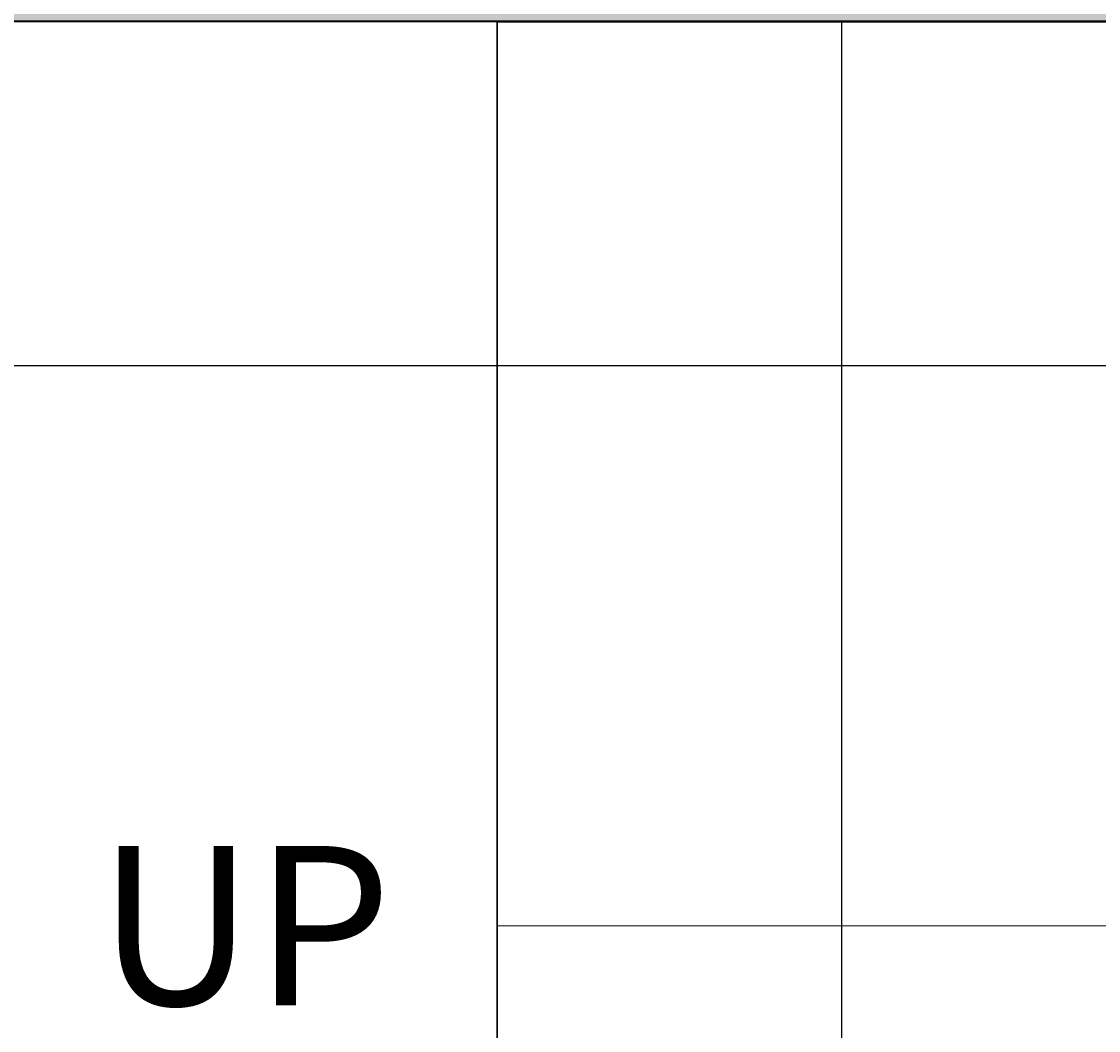
# Model space of a CAD drawing. Units: inches. Extents: x 1998 to 2588, y 1139 to 1977.
# Tile 106 of 134: x 2397 to 2422, y 1613 to 1637. Entities that reach past the tile are written whole.
import ezdxf

# ---------------------------------------------------------------- set-up
doc = ezdxf.new("R2010")
doc.units = ezdxf.units.IN
for name, color, linetype, lineweight in [('A-ANNO-DIMS', 2, 'Continuous', 18), ('A-ANNO-SYMB', 7, 'Continuous', 18), ('A-FLOR-STRS', 7, 'Continuous', 25), ('A-WALL-PATT', 252, 'Continuous', 13), ('WALL', 200, 'Continuous', 35)]:
    doc.layers.add(name, color=color, linetype=linetype, lineweight=lineweight)
doc.styles.get("Standard").update_dxf_attribs({"font": 'arial.ttf'})
doc.dimstyles.get("Standard").update_dxf_attribs({"dimtxt": 0.18, "dimasz": 0.18, "dimexe": 0.18, "dimexo": 0.0625, "dimgap": 0.09, "dimtad": 0, "dimtih": 1, "dimtoh": 1, "dimdec": 4, "dimzin": 0, "dimdsep": 46, "dimtxsty": 'Standard', "dimcen": 0.09, "dimadec": 0, "dimazin": 0, "dimtfac": 1, "dimtdec": 4, "dimtofl": 0, "dimtmove": 0, "dimatfit": 3, "dimfxl": 1, "dimtolj": 1, "dimtzin": 0, "dimarcsym": 0})

# ---------------------------------------------------------------- blocks, each defined once
blk = doc.blocks.new('*D24')
at = {"layer": 'A-ANNO-DIMS', "color": 0, "lineweight": -2, "transparency": 16777216}
for p, q in [((2398.535, 1911.232), (2588.309, 1911.232)), ((2588.129, 1911.052), (2588.129, 1570.164)), ((2588.129, 1228.912), (2588.129, 1569.8)), ((2527.535, 1228.732), (2588.309, 1228.732))]:
    blk.add_line(p, q, dxfattribs=at)
at = {"layer": 'A-ANNO-DIMS', "color": 0, "transparency": 16777216}
for points in [[(2588.099, 1911.052), (2588.159, 1911.052), (2588.129, 1911.232)], [(2588.099, 1228.912), (2588.159, 1228.912), (2588.129, 1228.732)]]:
    blk.add_solid(points, dxfattribs=at)
at = {"layer": 'Defpoints', "color": 0, "transparency": 16777216}
for p in [(2398.473, 1911.232), (2588.129, 1911.232), (2527.473, 1228.732)]:
    blk.add_point(p, dxfattribs=at)
at = {"layer": 'A-ANNO-DIMS', "color": 0, "transparency": 16777216, "insert": (2588.129, 1569.982), "char_height": 0.18, "attachment_point": 5}
blk.add_mtext('\\A1;682.5', dxfattribs=at)
blk = doc.blocks.new('*D30')
at = {"layer": 'A-ANNO-DIMS', "color": 0, "lineweight": -2, "transparency": 16777216}
for p, q in [((2407.91, 1636.732), (1997.843, 1636.732)), ((1998.023, 1636.552), (1998.023, 1615.913)), ((1998.023, 1594.912), (1998.023, 1615.552)), ((2407.91, 1594.732), (1997.843, 1594.732))]:
    blk.add_line(p, q, dxfattribs=at)
at = {"layer": 'A-ANNO-DIMS', "color": 0, "transparency": 16777216}
for points in [[(1997.993, 1636.552), (1998.053, 1636.552), (1998.023, 1636.732)], [(1997.993, 1594.912), (1998.053, 1594.912), (1998.023, 1594.732)]]:
    blk.add_solid(points, dxfattribs=at)
at = {"layer": 'Defpoints', "color": 0, "transparency": 16777216}
for p in [(1998.023, 1636.732), (2407.973, 1636.732), (2407.973, 1594.732)]:
    blk.add_point(p, dxfattribs=at)
at = {"layer": 'A-ANNO-DIMS', "color": 0, "transparency": 16777216, "insert": (1998.023, 1615.732), "char_height": 0.18, "attachment_point": 5}
blk.add_mtext('\\A1;42', dxfattribs=at)
blk = doc.blocks.new('*D39')
at = {"layer": 'A-ANNO-DIMS', "color": 0, "lineweight": -2, "transparency": 16777216}
for p, q in [((2115.035, 1628.742), (2588.309, 1628.742)), ((2588.129, 1628.562), (2588.129, 1612.685)), ((2588.129, 1596.444), (2588.129, 1612.321)), ((2115.035, 1596.264), (2588.309, 1596.264))]:
    blk.add_line(p, q, dxfattribs=at)
at = {"layer": 'A-ANNO-DIMS', "color": 0, "transparency": 16777216}
for points in [[(2588.099, 1628.562), (2588.159, 1628.562), (2588.129, 1628.742)], [(2588.099, 1596.444), (2588.159, 1596.444), (2588.129, 1596.264)]]:
    blk.add_solid(points, dxfattribs=at)
at = {"layer": 'Defpoints', "color": 0, "transparency": 16777216}
for p in [(2114.973, 1628.742), (2588.129, 1628.742), (2114.973, 1596.264)]:
    blk.add_point(p, dxfattribs=at)
at = {"layer": 'A-ANNO-DIMS', "color": 0, "transparency": 16777216, "insert": (2588.129, 1612.503), "char_height": 0.18, "attachment_point": 5}
blk.add_mtext('\\A1;32.48', dxfattribs=at)

msp = doc.modelspace()

# ---------------------------------------------------------------- hatches: boundary and pattern name
at = {"layer": 'A-WALL-PATT'}
h = msp.add_hatch(color=256, dxfattribs=at)
h.dxf.hatch_style = 1
h.paths.add_polyline_path([(2527.4729, 1362.2324), (2510.9729, 1362.2324), (2510.9729, 1357.7324), (2518.4729, 1357.7324), (2518.4729, 1237.7324), (2503.1458, 1237.7324), (2503.1458, 1228.7324), (2527.4729, 1228.7324)])
h.paths.add_polyline_path([(2490.5682, 1362.2324), (2398.4729, 1362.2324), (2398.4729, 1357.7324), (2490.5682, 1357.7324)])
h.paths.add_polyline_path([(2224.9729, 1264.7324), (2222.9729, 1264.7324), (2222.9729, 1232.4125), (2341.4729, 1232.4125), (2341.4729, 1234.4125), (2224.9729, 1234.4125)])
h.paths.add_polyline_path([(2334.5332, 1273.7324), (2264.7638, 1273.7324), (2264.7638, 1269.5611, -0.043659), (2264.3413, 1264.7324), (2334.5332, 1264.7324)])
h.paths.add_polyline_path([(2236.9551, 1273.7324), (2234.4125, 1273.7324), (2234.4125, 1264.7324), (2236.9551, 1264.7324), (2236.9551, 1269.5611)])
h.paths.add_polyline_path([(2222.9729, 1293.2324), (2096.9729, 1293.2324), (2096.9729, 1345.0966), (2087.9729, 1345.0966), (2087.9729, 1284.2324), (2222.9729, 1284.2324), (2222.9729, 1285.137)])
h.paths.add_polyline_path([(2096.9729, 1458.7927), (2087.9729, 1458.7927), (2087.9729, 1417.7324), (2087.9729, 1413.2324), (2096.9729, 1413.2324), (2096.9729, 1417.7324)])
h.paths.add_polyline_path([(2096.9729, 1413.2324), (2087.9729, 1413.2324), (2087.9729, 1365.5012), (2096.9729, 1365.5012), (2096.9729, 1369.3358)])
h.paths.add_polyline_path([(2186.2943, 1417.7324), (2138.6074, 1417.7324), (2096.9729, 1417.7324), (2096.9729, 1413.2324), (2138.6074, 1413.2324), (2186.2943, 1413.2324)])
h.paths.add_polyline_path([(2181.4729, 1465.7324), (2176.9729, 1465.7324), (2176.9729, 1451.6434), (2181.4729, 1451.6434)])
h.paths.add_polyline_path([(2181.4729, 1422.1664), (2176.9729, 1422.1664), (2176.9729, 1417.7324), (2181.4729, 1417.7324)])
h.paths.add_polyline_path([(2063.9729, 1465.7324), (2087.9729, 1465.7324), (2087.9729, 1470.2324), (2059.4729, 1470.2324), (2059.4729, 1413.2324), (2087.9729, 1413.2324), (2087.9729, 1417.7324), (2063.9729, 1417.7324)])
h.paths.add_polyline_path([(2181.4729, 1755.2324), (2176.9729, 1755.2324), (2176.9729, 1748.6798), (2177.0513, 1748.6798), (2181.4729, 1748.6798)])
h.paths.add_polyline_path([(2227.4729, 1707.2324), (2220.4647, 1707.2324), (2220.4647, 1702.7324), (2222.9729, 1702.7324), (2222.9729, 1604.637), (2227.4729, 1604.637)])
h.paths.add_polyline_path([(2114.9729, 1702.7324), (2105.9729, 1702.7324), (2105.9729, 1628.4781, -0.0318759), (2110.1012, 1628.7416), (2114.9729, 1628.7416)])
h.paths.add_polyline_path([(2345.9729, 1739.3278), (2341.4729, 1739.3278), (2341.4729, 1647.5211), (2345.9729, 1647.5211)])
h.paths.add_polyline_path([(2350.6273, 1641.2324), (2345.9729, 1641.2324), (2345.9729, 1636.7324), (2350.6273, 1636.7324), (2350.6273, 1639.8729)])
h.paths.add_polyline_path([(2501.9729, 1641.2324), (2407.9729, 1641.2324), (2392.5005, 1641.2324), (2392.5005, 1639.8729), (2392.5005, 1636.7324), (2501.9729, 1636.7324)])
h.paths.add_polyline_path([(2510.9729, 1755.2324), (2501.9729, 1755.2324), (2501.9729, 1641.2324), (2510.9729, 1641.2324)])
h.paths.add_polyline_path([(2549.1786, 1641.2324), (2522.3775, 1641.2324), (2522.3775, 1636.7324), (2540.1786, 1636.7324), (2540.1786, 1480.7324), (2522.3775, 1480.7324), (2522.3775, 1476.2324), (2549.1786, 1476.2324)])
h.paths.add_polyline_path([(2498.1786, 1594.7324), (2407.9729, 1594.7324), (2407.9729, 1585.7324), (2416.9729, 1585.7324), (2489.1786, 1585.7324), (2489.1786, 1531.7324), (2416.9729, 1531.7324), (2407.9729, 1531.7324), (2407.9729, 1522.7324), (2498.1786, 1522.7324)])
h.paths.add_polyline_path([(2351.6437, 1480.7324), (2345.9729, 1480.7324), (2345.9729, 1476.2324), (2351.6437, 1476.2324), (2351.6437, 1477.5919)])
h.paths.add_polyline_path([(2501.9729, 1480.7324), (2498.1786, 1480.7324), (2407.9729, 1480.7324), (2393.5168, 1480.7324), (2393.5168, 1477.5919), (2393.5168, 1476.2324), (2501.9729, 1476.2324)])

# ---------------------------------------------------------------- linework, layer by layer
at = {"layer": 'A-ANNO-SYMB'}
msp.add_line((2407.9729, 1615.7324), (2505.7676, 1615.7324), dxfattribs=at)
at = {"layer": 'A-FLOR-STRS'}
for p, q in [((2407.9729, 1480.7324), (2407.9729, 1636.7324)), ((2407.9729, 1636.7324), (2407.9729, 1594.7324)), ((2415.9729, 1636.7324), (2415.9729, 1594.7324))]:
    msp.add_line(p, q, dxfattribs=at)
at = {"layer": 'WALL'}
for p, q in [((2501.9729, 1636.7324), (2392.5005, 1636.7324)), ((2407.9729, 1636.7324), (2501.9729, 1636.7324))]:
    msp.add_line(p, q, dxfattribs=at)

# ---------------------------------------------------------------- texts
at = {"layer": 'A-ANNO-SYMB', "insert": (2398.6914, 1617.5871), "char_height": 3.69875, "attachment_point": 1}
msp.add_mtext_dynamic_manual_height_columns('UP', width=110.572713, gutter_width=18.4938, heights=[0], dxfattribs=at)

# ---------------------------------------------------------------- dimensions: what is measured, and where the dimension line sits
at = {"layer": 'A-ANNO-DIMS'}
for base, p1, p2, override, picture, middle in [((2588.1286, 1911.2324), (2527.4729, 1228.7324), (2398.4729, 1911.2324), {"dimdec": 1, "dimlfac": 1, "dimrnd": 0, "dimzin": 0, "dimdsep": 46, "dimlunit": 2}, '*D24', (2588.1286, 1569.9824)), ((1998.0229, 1636.7324), (2407.9729, 1594.7324), (2407.9729, 1636.7324), {"dimdec": 0, "dimlfac": 1, "dimrnd": 0, "dimzin": 0, "dimdsep": 46, "dimlunit": 2}, '*D30', (1998.0229, 1615.7324)), ((2588.1286, 1628.7416), (2114.9729, 1596.2642), (2114.9729, 1628.7416), {"dimdec": 2, "dimlfac": 1, "dimrnd": 0, "dimzin": 0, "dimdsep": 46, "dimlunit": 2}, '*D39', (2588.1286, 1612.5029))]:
    dim = msp.add_linear_dim(base=base, p1=p1, p2=p2, angle=90, dimstyle='Standard', override=override, dxfattribs=at)
    dim.commit()
    dim.dimension.update_dxf_attribs({"geometry": picture, "text_midpoint": middle})

doc.saveas('drawing.dxf')
